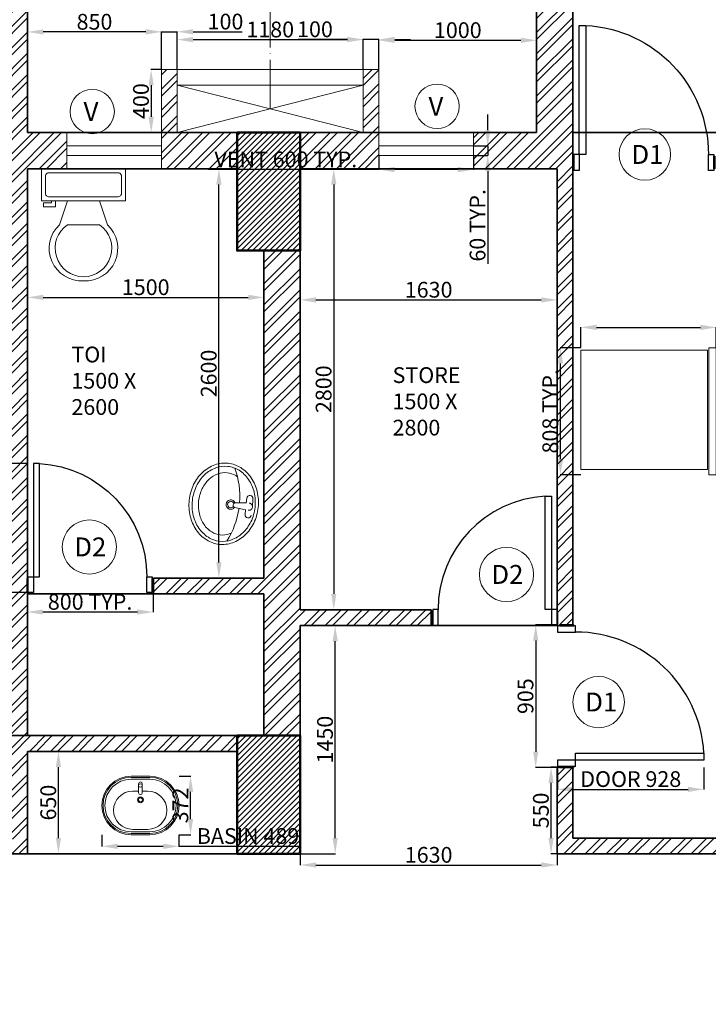
# Model space of a CAD drawing. Units: millimetres. Extents: x -3326 to 29338, y -16792 to 6002.
# Tile 9 of 21: x 3793 to 8162, y -3440 to 2813. Entities that reach past the tile are written whole.
import ezdxf

# ---------------------------------------------------------------- set-up
doc = ezdxf.new("R2010")
doc.units = ezdxf.units.MM
doc.header["$PDMODE"] = 35
doc.header["$PDSIZE"] = 5
doc.linetypes.add('ACAD_ISO04W100', pattern=[30, 24, -3, 0, -3])
for name, color, linetype, lineweight in [('A-ANNO-DIMS', 2, 'Continuous', 13), ('A-ANNO-SYMB', 7, 'Continuous', 18), ('A-AREA-IDEN', 7, 'Continuous', 18), ('A-COLS', 1, 'Continuous', 50), ('A-COLS-PATT', 251, 'Continuous', 13), ('A-DOOR', 3, 'Continuous', 25), ('A-EQPM', 9, 'Continuous', 18), ('A-FLOR-FIXT', 9, 'Continuous', 18), ('A-FLOR-SHFT', 8, 'Continuous', 18), ('A-GLAZ', 4, 'Continuous', 18), ('A-GRID', 8, 'ACAD_ISO04W100', 13), ('A-WALL', 7, 'Continuous', 35), ('A-WALL-PATT', 252, 'Continuous', 13)]:
    doc.layers.add(name, color=color, linetype=linetype, lineweight=lineweight)
doc.styles.get("Standard").update_dxf_attribs({"font": 'arial.ttf'})
doc.dimstyles.new('ISO-25', dxfattribs={"dimtxt": 100, "dimasz": 100, "dimexe": 1.25, "dimexo": 0.625, "dimtad": 1, "dimtxsty": 'Standard', "dimcen": 2.5, "dimadec": 0, "dimazin": 0, "dimtfac": 1, "dimtmove": 0, "dimatfit": 3, "dimfxl": 1, "dimarcsym": 0})
pattern_1 = [(45, (-10476.65, 1e-12), (-67.35192, 67.35192), []), (45, (-10431.74, 1e-12), (-67.35192, 67.35192), [])]

# ---------------------------------------------------------------- blocks, each defined once
blk = doc.blocks.new('A$C6ED17C1F')
for points in [[(793.9, 100), (720, 100), (720, 820), (760, 820), (760, 0), (793.9, 0)], [(6.1, 0), (40, 0), (40, 100), (6.1, 100)], [(6.1, 100), (6.1, 0)], [(793.9, 100), (793.9, 0)]]:
    blk.add_lwpolyline(points)
for points in [[(0, 10), (6.1, 10), (6.1, 90), (0, 90)], [(793.9, 10), (800, 10), (800, 90), (793.9, 90)]]:
    blk.add_lwpolyline(points, close=True)
blk.add_arc((761.2, 100), 721.2, 93.2732, 180)
blk = doc.blocks.new('A$C0CE462CD')
for p, q in [((860, 100), (860, 0)), ((860, 0), (893.9, 0))]:
    blk.add_line(p, q)
for points in [[(860, 100), (860, 920), (818.4, 920), (818.4, 100)], [(0, 10), (6.1, 10), (6.1, 90), (0, 90)], [(893.9, 10), (900, 10), (900, 90), (893.9, 90)]]:
    blk.add_lwpolyline(points, close=True)
for points in [[(6.1, 0), (40, 0), (40, 100), (6.1, 100)], [(6.1, 100), (6.1, 0)], [(860, 100), (893.9, 100), (893.9, 0)]]:
    blk.add_lwpolyline(points)
blk.add_arc((859.1, 101.9), 819.1, 92.8508, 180.13091)
blk = doc.blocks.new('*U5')
for p, q in [((9.5, -6), (9.5, -2)), ((-10, -8.5), (-8, -8.5)), ((-10, -9.5), (-10, -8.5)), ((-7, -9.5), (-10, -9.5)), ((-8, -8.5), (-8, -8)), ((-7, -8), (-7, -9.5)), ((-4, -8), (-6, -14)), ((4, -8), (6, -14)), ((4, -14), (-4, -14))]:
    blk.add_line(p, q)
blk.add_lwpolyline([(10.5, -8), (10.5, 0), (-10.5, 0), (-10.5, -8)], close=True)
for points in [[(-9.5, -2), (-9.5, -6)], [(8.5, -1), (-8.5, -1)], [(-8.5, -7), (8.5, -7)]]:
    blk.add_lwpolyline(points)
for centre, radius, start, end in [((-8.625, -1.875), 0.8839, 81.8699, 188.1301), ((8.625, -1.875), 0.8839, 351.8699, 98.1301), ((-8.625, -6.125), 0.8839, 171.869898, 278.1301), ((8.625, -6.125), 0.8839, 261.8699, 8.1301), ((-0.4772, -19.9188), 8.0953, 133.01722, 273.38), ((0.0374, -19.8731), 7.127, 124.50543, 269.7), ((-0.0373, -19.8731), 7.127, 270.3, 55.4946), ((0.4773, -19.9188), 8.0953, 266.62, 46.9828)]:
    blk.add_arc(centre, radius, start, end)
blk = doc.blocks.new('A$C6B943AC5')
for p, q in [((0.207, 0.401), (0.2589, 0.4042)), ((0.2071, 0.362), (0.2386, 0.3621)), ((0.2361, 0.3625), (0.2439, 0.2926)), ((0.2809, 0.3627), (0.2736, 0.2927)), ((0.3111, 0.3624), (0.2796, 0.3623))]:
    blk.add_line(p, q)
for points in [[(0.518, 0.2209, -0.113917), (0.4993, 0.1385, -0.1036), (0.4427, 0.0651, -0.091717), (0.3606, 0.0176, -0.084781), (0.2598, 0, -0.084781), (0.1587, 0.0169, -0.091717), (0.0764, 0.0638, -0.1036), (0.0193, 0.1368, -0.113917), (0, 0.2191, -0.113917), (0.0187, 0.3015, -0.1036), (0.0753, 0.3749, -0.091717), (0.1574, 0.4224, -0.084781), (0.2582, 0.44, -0.084781), (0.3592, 0.4231, -0.091717), (0.4416, 0.3762, -0.1036), (0.4987, 0.3032, -0.113917)], [(0.498, 0.2208, -0.113917), (0.4813, 0.1472, -0.1036), (0.4297, 0.0803, -0.091717), (0.3539, 0.0364, -0.084781), (0.2597, 0.02, -0.084781), (0.1653, 0.0358, -0.091717), (0.0893, 0.0791, -0.1036), (0.0372, 0.1457, -0.113917), (0.02, 0.2192, -0.113917), (0.0367, 0.2928, -0.1036), (0.0883, 0.3597, -0.091717), (0.1641, 0.4036, -0.084781), (0.2583, 0.42, -0.084781), (0.3527, 0.4042, -0.091717), (0.4287, 0.3609, -0.1036), (0.4808, 0.2943, -0.113917)]]:
    blk.add_lwpolyline(points, format="xyb", close=True)
for points in [[(0.458, 0.2207, -0.113917), (0.4453, 0.1646, -0.1036), (0.4037, 0.1107, -0.091717), (0.3405, 0.0741, -0.084781), (0.2595, 0.06, -0.084781), (0.1785, 0.0736, -0.091717), (0.1151, 0.1097, -0.1036), (0.0731, 0.1633, -0.113917), (0.06, 0.2193, -0.113917), (0.0727, 0.2754, -0.020517), (0.0792, 0.2874, -0.091717)], [(0.4384, 0.2886, -0.020517), (0.4449, 0.2767, -0.113917), (0.458, 0.2207, -0.113917)]]:
    blk.add_lwpolyline(points, format="xyb")
for centre, radius, start, end in [((0.207, 0.3815), 0.0195, 90.19698, 270.19698), ((0.259, 0.3817), 0.0225, 354.08148, 186.31248), ((0.311, 0.3819), 0.0195, 270.19698, 90.19698), ((0.2604, -0.2004), 0.5204, 92.15427, 116.77617), ((0.2604, -0.2004), 0.5204, 63.61779, 88.23969), ((0.2588, 0.265), 0.03, 119.152, 61.24195), ((0.2588, 0.265), 0.02, 116.58131, 63.81265), ((0.2587, 0.295), 0.015, 189.39225, 351.00171)]:
    blk.add_arc(centre, radius, start, end)
blk = doc.blocks.new('A$C6AF055E0')
for p, q in [((0.1999, 0.245), (0.1225, 0.245)), ((0.1999, 0.24), (0.1225, 0.24)), ((0.1999, 0.2325), (0.1225, 0.2325)), ((0.1537, 0.1758), (0.1537, 0.2135)), ((0.1687, 0.2135), (0.1687, 0.1758)), ((0.129, 0.1825), (0.1537, 0.1825)), ((0.1687, 0.1825), (0.1919, 0.1825)), ((0.1225, 0.0125), (0.1999, 0.0125)), ((0.1225, 0.005), (0.1999, 0.005)), ((0.1225, 0), (0.1999, 0)), ((0.129, 0.0225), (0.1919, 0.0225))]:
    blk.add_line(p, q)
for centre, radius in [((0.1612, 0.206), 0.0075), ((0.1612, 0.1463), 0.0125), ((0.1612, 0.1463), 0.0085)]:
    blk.add_circle(centre, radius)
for centre, radius, start, end in [((0.1225, 0.1225), 0.1225, 90, 270), ((0.1225, 0.1225), 0.1175, 90, 270), ((0.1225, 0.1225), 0.11, 90, 270), ((0.1612, 0.2135), 0.0075, 0, 180), ((0.1999, 0.1225), 0.1225, 270, 90), ((0.1999, 0.1225), 0.1175, 270, 90), ((0.1999, 0.1225), 0.11, 270, 90), ((0.129, 0.1025), 0.08, 90, 270), ((0.1612, 0.1758), 0.0075, 180, 0), ((0.1919, 0.1025), 0.08, 270, 90)]:
    blk.add_arc(centre, radius, start, end)
blk = doc.blocks.new('*D128')
at = {"layer": 'A-ANNO-DIMS', "color": 0, "lineweight": -2, "transparency": 16777216}
for p, q in [((5572.3, 1033.9), (5572.3, 1034.6)), ((5672.3, 1033.3), (7102.3, 1033.3)), ((7202.3, 1033.9), (7202.3, 1034.6))]:
    blk.add_line(p, q, dxfattribs=at)
at = {"layer": 'A-ANNO-DIMS', "color": 0, "transparency": 16777216}
for points in [[(5672.3, 1050), (5672.3, 1016.6), (5572.3, 1033.3)], [(7102.3, 1050), (7102.3, 1016.6), (7202.3, 1033.3)]]:
    blk.add_solid(points, dxfattribs=at)
at = {"layer": 'Defpoints', "color": 0, "transparency": 16777216}
for p in [(5572.3, 1033.3), (7202.3, 1033.3), (7202.3, 1033.3)]:
    blk.add_point(p, dxfattribs=at)
at = {"layer": 'A-ANNO-DIMS', "color": 0, "transparency": 16777216, "insert": (6387.3, 1085), "char_height": 100, "attachment_point": 5}
blk.add_mtext('1630', dxfattribs=at)
blk = doc.blocks.new('*D129')
at = {"layer": 'A-ANNO-DIMS', "color": 0, "lineweight": -2, "transparency": 16777216}
for p, q in [((5572.9, 1866), (5786.7, 1866)), ((5785.5, 1766), (5785.5, -834)), ((5572.9, -934), (5786.7, -934))]:
    blk.add_line(p, q, dxfattribs=at)
at = {"layer": 'A-ANNO-DIMS', "color": 0, "transparency": 16777216}
for points in [[(5768.8, 1766), (5802.1, 1766), (5785.5, 1866)], [(5768.8, -834), (5802.1, -834), (5785.5, -934)]]:
    blk.add_solid(points, dxfattribs=at)
at = {"layer": 'Defpoints', "color": 0, "transparency": 16777216}
for p in [(5572.3, 1866), (5572.3, -934), (5785.5, -934)]:
    blk.add_point(p, dxfattribs=at)
at = {"layer": 'A-ANNO-DIMS', "color": 0, "transparency": 16777216, "insert": (5733.8, 466), "char_height": 100, "attachment_point": 5, "rotation": 90}
blk.add_mtext('2800', dxfattribs=at)
blk = doc.blocks.new('*D130')
at = {"layer": 'A-ANNO-DIMS', "color": 0, "lineweight": -2, "transparency": 16777216}
for p, q in [((3842.3, 1103.3), (3842.3, 1048.1)), ((5342.3, 1103.3), (5342.3, 1048.1)), ((3942.3, 1049.4), (5242.3, 1049.4))]:
    blk.add_line(p, q, dxfattribs=at)
at = {"layer": 'A-ANNO-DIMS', "color": 0, "transparency": 16777216}
for points in [[(3942.3, 1066), (3942.3, 1032.7), (3842.3, 1049.4)], [(5242.3, 1066), (5242.3, 1032.7), (5342.3, 1049.4)]]:
    blk.add_solid(points, dxfattribs=at)
at = {"layer": 'Defpoints', "color": 0, "transparency": 16777216}
for p in [(3842.3, 1103.9), (5342.3, 1103.9), (5342.3, 1049.4)]:
    blk.add_point(p, dxfattribs=at)
at = {"layer": 'A-ANNO-DIMS', "color": 0, "transparency": 16777216, "insert": (4592.3, 1101.1), "char_height": 100, "attachment_point": 5}
blk.add_mtext('1500', dxfattribs=at)
blk = doc.blocks.new('*D131')
at = {"layer": 'A-ANNO-DIMS', "color": 0, "lineweight": -2, "transparency": 16777216}
for p, q in [((5171.7, 1866), (5055.3, 1866)), ((5056.6, -634), (5056.6, 1766)), ((5341.7, -734), (5055.3, -734))]:
    blk.add_line(p, q, dxfattribs=at)
at = {"layer": 'A-ANNO-DIMS', "color": 0, "transparency": 16777216}
for points in [[(5039.9, 1766), (5073.2, 1766), (5056.6, 1866)], [(5039.9, -634), (5073.2, -634), (5056.6, -734)]]:
    blk.add_solid(points, dxfattribs=at)
at = {"layer": 'Defpoints', "color": 0, "transparency": 16777216}
for p in [(5056.6, 1866), (5172.3, 1866), (5342.3, -734)]:
    blk.add_point(p, dxfattribs=at)
at = {"layer": 'A-ANNO-DIMS', "color": 0, "transparency": 16777216, "insert": (5004.9, 566), "char_height": 100, "attachment_point": 5, "rotation": 90}
blk.add_mtext('2600', dxfattribs=at)
blk = doc.blocks.new('*D132')
at = {"layer": 'A-ANNO-DIMS', "color": 0, "lineweight": -2, "transparency": 16777216}
for p, q in [((5572.9, -1034), (5795.7, -1034)), ((5794.4, -2384), (5794.4, -1134)), ((5572.9, -2484), (5795.7, -2484))]:
    blk.add_line(p, q, dxfattribs=at)
at = {"layer": 'A-ANNO-DIMS', "color": 0, "transparency": 16777216}
for points in [[(5777.8, -1134), (5811.1, -1134), (5794.4, -1034)], [(5777.8, -2384), (5811.1, -2384), (5794.4, -2484)]]:
    blk.add_solid(points, dxfattribs=at)
at = {"layer": 'Defpoints', "color": 0, "transparency": 16777216}
for p in [(5572.3, -1034), (5794.4, -1034), (5572.3, -2484)]:
    blk.add_point(p, dxfattribs=at)
at = {"layer": 'A-ANNO-DIMS', "color": 0, "transparency": 16777216, "insert": (5742.8, -1759), "char_height": 100, "attachment_point": 5, "rotation": 90}
blk.add_mtext('1450', dxfattribs=at)
blk = doc.blocks.new('*D133')
at = {"layer": 'A-ANNO-DIMS', "color": 0, "lineweight": -2, "transparency": 16777216}
for p, q in [((7201.7, -1934), (7162.8, -1934)), ((7164.1, -2384), (7164.1, -2034)), ((7201.7, -2484), (7162.8, -2484))]:
    blk.add_line(p, q, dxfattribs=at)
at = {"layer": 'A-ANNO-DIMS', "color": 0, "transparency": 16777216}
for points in [[(7147.4, -2034), (7180.7, -2034), (7164.1, -1934)], [(7147.4, -2384), (7180.7, -2384), (7164.1, -2484)]]:
    blk.add_solid(points, dxfattribs=at)
at = {"layer": 'Defpoints', "color": 0, "transparency": 16777216}
for p in [(7164.1, -1934), (7202.3, -1934), (7202.3, -2484)]:
    blk.add_point(p, dxfattribs=at)
at = {"layer": 'A-ANNO-DIMS', "color": 0, "transparency": 16777216, "insert": (7112.4, -2209), "char_height": 100, "attachment_point": 5, "rotation": 90}
blk.add_mtext('550', dxfattribs=at)
blk = doc.blocks.new('*D134')
at = {"layer": 'A-ANNO-DIMS', "color": 0, "lineweight": -2, "transparency": 16777216}
for p, q in [((5572.3, -2484.6), (5572.3, -2556.8)), ((7202.3, -2484.6), (7202.3, -2556.8)), ((5672.3, -2555.5), (7102.3, -2555.5))]:
    blk.add_line(p, q, dxfattribs=at)
at = {"layer": 'A-ANNO-DIMS', "color": 0, "transparency": 16777216}
for points in [[(5672.3, -2538.9), (5672.3, -2572.2), (5572.3, -2555.5)], [(7102.3, -2538.9), (7102.3, -2572.2), (7202.3, -2555.5)]]:
    blk.add_solid(points, dxfattribs=at)
at = {"layer": 'Defpoints', "color": 0, "transparency": 16777216}
for p in [(5572.3, -2484), (7202.3, -2484), (7202.3, -2555.5)]:
    blk.add_point(p, dxfattribs=at)
at = {"layer": 'A-ANNO-DIMS', "color": 0, "transparency": 16777216, "insert": (6387.3, -2503.8), "char_height": 100, "attachment_point": 5}
blk.add_mtext('1630', dxfattribs=at)
blk = doc.blocks.new('*D135')
at = {"layer": 'A-ANNO-DIMS', "color": 0, "lineweight": -2, "transparency": 16777216}
for p, q in [((3842.9, -1834), (4039.8, -1834)), ((4038.5, -2384), (4038.5, -1934)), ((3842.9, -2484), (4039.8, -2484))]:
    blk.add_line(p, q, dxfattribs=at)
at = {"layer": 'A-ANNO-DIMS', "color": 0, "transparency": 16777216}
for points in [[(4021.9, -1934), (4055.2, -1934), (4038.5, -1834)], [(4021.9, -2384), (4055.2, -2384), (4038.5, -2484)]]:
    blk.add_solid(points, dxfattribs=at)
at = {"layer": 'Defpoints', "color": 0, "transparency": 16777216}
for p in [(3842.3, -1834), (4038.5, -1834), (3842.3, -2484)]:
    blk.add_point(p, dxfattribs=at)
at = {"layer": 'A-ANNO-DIMS', "color": 0, "transparency": 16777216, "insert": (3986.9, -2159), "char_height": 100, "attachment_point": 5, "rotation": 90}
blk.add_mtext('650', dxfattribs=at)
blk = doc.blocks.new('*D145')
at = {"layer": 'A-ANNO-DIMS', "color": 0, "lineweight": -2, "transparency": 16777216}
for p, q in [((4792.3, 2496.7), (4792.3, 2687.3)), ((4892.3, 2686.1), (5872.3, 2686.1)), ((5972.3, 2496.7), (5972.3, 2687.3))]:
    blk.add_line(p, q, dxfattribs=at)
at = {"layer": 'A-ANNO-DIMS', "color": 0, "transparency": 16777216}
for points in [[(4892.3, 2702.8), (4892.3, 2669.4), (4792.3, 2686.1)], [(5872.3, 2702.8), (5872.3, 2669.4), (5972.3, 2686.1)]]:
    blk.add_solid(points, dxfattribs=at)
at = {"layer": 'Defpoints', "color": 0, "transparency": 16777216}
for p in [(5972.3, 2686.1), (4792.3, 2496), (5972.3, 2496)]:
    blk.add_point(p, dxfattribs=at)
at = {"layer": 'A-ANNO-DIMS', "color": 0, "transparency": 16777216, "insert": (5382.3, 2737.8), "char_height": 100, "attachment_point": 5}
blk.add_mtext('1180', dxfattribs=at)
blk = doc.blocks.new('*D146')
at = {"layer": 'A-ANNO-DIMS', "color": 0, "lineweight": -2, "transparency": 16777216}
for p, q in [((4592.3, 2736.2), (4492.3, 2736.2)), ((4692.3, 2496.7), (4692.3, 2737.4)), ((4692.3, 2736.2), (4792.3, 2736.2)), ((4792.3, 2496.7), (4792.3, 2737.4)), ((4892.3, 2736.2), (5204.7, 2736.2))]:
    blk.add_line(p, q, dxfattribs=at)
at = {"layer": 'A-ANNO-DIMS', "color": 0, "transparency": 16777216}
for points in [[(4592.3, 2752.9), (4592.3, 2719.5), (4692.3, 2736.2)], [(4892.3, 2752.9), (4892.3, 2719.5), (4792.3, 2736.2)]]:
    blk.add_solid(points, dxfattribs=at)
at = {"layer": 'Defpoints', "color": 0, "transparency": 16777216}
for p in [(4792.3, 2736.2), (4692.3, 2496), (4792.3, 2496)]:
    blk.add_point(p, dxfattribs=at)
at = {"layer": 'A-ANNO-DIMS', "color": 0, "transparency": 16777216, "insert": (5098.5, 2787.9), "char_height": 100, "attachment_point": 5}
blk.add_mtext('100', dxfattribs=at)
blk = doc.blocks.new('*D147')
at = {"layer": 'A-ANNO-DIMS', "color": 0, "lineweight": -2, "transparency": 16777216}
for p, q in [((5872.3, 2687.3), (5559.9, 2687.3)), ((5972.3, 2496.7), (5972.3, 2688.6)), ((6072.3, 2687.3), (5972.3, 2687.3)), ((6072.3, 2496.7), (6072.3, 2688.6)), ((6172.3, 2687.3), (6272.3, 2687.3))]:
    blk.add_line(p, q, dxfattribs=at)
at = {"layer": 'A-ANNO-DIMS', "color": 0, "transparency": 16777216}
for points in [[(5872.3, 2704), (5872.3, 2670.7), (5972.3, 2687.3)], [(6172.3, 2704), (6172.3, 2670.7), (6072.3, 2687.3)]]:
    blk.add_solid(points, dxfattribs=at)
at = {"layer": 'Defpoints', "color": 0, "transparency": 16777216}
for p in [(5972.3, 2687.3), (5972.3, 2496), (6072.3, 2496)]:
    blk.add_point(p, dxfattribs=at)
at = {"layer": 'A-ANNO-DIMS', "color": 0, "transparency": 16777216, "insert": (5666.1, 2739), "char_height": 100, "attachment_point": 5}
blk.add_mtext('100', dxfattribs=at)
blk = doc.blocks.new('*D148')
at = {"layer": 'A-ANNO-DIMS', "color": 0, "lineweight": -2, "transparency": 16777216}
for p, q in [((6072.3, 2593.3), (6072.3, 2683)), ((6172.3, 2681.8), (6972.3, 2681.8)), ((7072.3, 2593.3), (7072.3, 2683))]:
    blk.add_line(p, q, dxfattribs=at)
at = {"layer": 'A-ANNO-DIMS', "color": 0, "transparency": 16777216}
for points in [[(6172.3, 2698.4), (6172.3, 2665.1), (6072.3, 2681.8)], [(6972.3, 2698.4), (6972.3, 2665.1), (7072.3, 2681.8)]]:
    blk.add_solid(points, dxfattribs=at)
at = {"layer": 'Defpoints', "color": 0, "transparency": 16777216}
for p in [(7072.3, 2681.8), (6072.3, 2592.6), (7072.3, 2592.6)]:
    blk.add_point(p, dxfattribs=at)
at = {"layer": 'A-ANNO-DIMS', "color": 0, "transparency": 16777216, "insert": (6572.3, 2733.4), "char_height": 100, "attachment_point": 5}
blk.add_mtext('1000', dxfattribs=at)
blk = doc.blocks.new('*D149')
at = {"layer": 'A-ANNO-DIMS', "color": 0, "lineweight": -2, "transparency": 16777216}
for p, q in [((3842.3, 2617.7), (3842.3, 2736.3)), ((4592.3, 2735), (3942.3, 2735)), ((4692.3, 2617.7), (4692.3, 2736.3))]:
    blk.add_line(p, q, dxfattribs=at)
at = {"layer": 'A-ANNO-DIMS', "color": 0, "transparency": 16777216}
for points in [[(3942.3, 2751.7), (3942.3, 2718.4), (3842.3, 2735)], [(4592.3, 2751.7), (4592.3, 2718.4), (4692.3, 2735)]]:
    blk.add_solid(points, dxfattribs=at)
at = {"layer": 'Defpoints', "color": 0, "transparency": 16777216}
for p in [(3842.3, 2735), (3842.3, 2617.1), (4692.3, 2617.1)]:
    blk.add_point(p, dxfattribs=at)
at = {"layer": 'A-ANNO-DIMS', "color": 0, "transparency": 16777216, "insert": (4267.3, 2786.7), "char_height": 100, "attachment_point": 5}
blk.add_mtext('850', dxfattribs=at)
blk = doc.blocks.new('*D150')
at = {"layer": 'A-ANNO-DIMS', "color": 0, "lineweight": -2, "transparency": 16777216}
for p, q in [((4691.7, 2496), (4625.5, 2496)), ((4626.8, 2396), (4626.8, 2196)), ((4691.7, 2096), (4625.5, 2096))]:
    blk.add_line(p, q, dxfattribs=at)
at = {"layer": 'A-ANNO-DIMS', "color": 0, "transparency": 16777216}
for points in [[(4610.1, 2396), (4643.5, 2396), (4626.8, 2496)], [(4610.1, 2196), (4643.5, 2196), (4626.8, 2096)]]:
    blk.add_solid(points, dxfattribs=at)
at = {"layer": 'Defpoints', "color": 0, "transparency": 16777216}
for p in [(4692.3, 2496), (4626.8, 2096), (4692.3, 2096)]:
    blk.add_point(p, dxfattribs=at)
at = {"layer": 'A-ANNO-DIMS', "color": 0, "transparency": 16777216, "insert": (4575.1, 2296), "char_height": 100, "attachment_point": 5, "rotation": 90}
blk.add_mtext('400', dxfattribs=at)
blk = doc.blocks.new('REFRIGERATOR-PLAN')
for points in [[(0, 791.3), (804.9, 791.3), (804.9, 34.9), (0, 34.9)], [(812.5, 807.8), (859.3, 807.8), (859.3, 0), (812.5, 0)]]:
    blk.add_lwpolyline(points, close=True)
blk = doc.blocks.new('TAG-D1')
blk.add_circle((163.3, 163.3), 163.3)
at = {"insert": (78, 223.5), "char_height": 120, "attachment_point": 1}
blk.add_mtext_dynamic_manual_height_columns('D1', width=137.943, gutter_width=12.5, heights=[0], dxfattribs=at)
blk = doc.blocks.new('TAG-D2')
blk.add_circle((172, 172), 172)
at = {"insert": (75.7, 232.2), "char_height": 120, "attachment_point": 1}
blk.add_mtext_dynamic_manual_height_columns('D2', width=130.724, gutter_width=12.5, heights=[0], dxfattribs=at)
blk = doc.blocks.new('TAG-V')
blk.add_circle((140.7, 140.7), 140.7)
at = {"insert": (85.8, 200.7), "char_height": 120, "attachment_point": 1}
blk.add_mtext_dynamic_manual_height_columns('V', width=129.836, gutter_width=12.5, heights=[0], dxfattribs=at)
blk = doc.blocks.new('GLAZ-600x60')
for p, q in [((0, 60), (600, 60)), ((0, 0), (600, 0))]:
    blk.add_line(p, q)
blk = doc.blocks.new('*D197')
at = {"layer": 'A-ANNO-DIMS', "color": 0, "lineweight": -2, "transparency": 16777216}
for p, q in [((3716.3, -5.8), (3716.3, 1112.9)), ((3838.6, -5.8), (3715, -5.8)), ((3716.3, -725.8), (3716.3, -105.8)), ((3838.6, -825.8), (3715, -825.8))]:
    blk.add_line(p, q, dxfattribs=at)
at = {"layer": 'A-ANNO-DIMS', "color": 0, "transparency": 16777216}
for points in [[(3699.6, -105.8), (3732.9, -105.8), (3716.3, -5.8)], [(3699.6, -725.8), (3732.9, -725.8), (3716.3, -825.8)]]:
    blk.add_solid(points, dxfattribs=at)
at = {"layer": 'Defpoints', "color": 0, "transparency": 16777216}
for p in [(3716.3, -5.8), (3839.3, -5.8), (3839.3, -825.8)]:
    blk.add_point(p, dxfattribs=at)
at = {"layer": 'A-ANNO-DIMS', "color": 0, "transparency": 16777216, "insert": (3663.9, 603.5), "char_height": 100, "attachment_point": 5, "rotation": 90}
blk.add_mtext('DOOR 820 TYP.', dxfattribs=at)
blk = doc.blocks.new('*D198')
at = {"layer": 'A-ANNO-DIMS', "color": 0, "lineweight": -2, "transparency": 16777216}
for p, q in [((3839.3, -826.4), (3839.3, -950)), ((4639.3, -826.4), (4639.3, -950)), ((4539.3, -948.8), (3939.3, -948.8))]:
    blk.add_line(p, q, dxfattribs=at)
at = {"layer": 'A-ANNO-DIMS', "color": 0, "transparency": 16777216}
for points in [[(3939.3, -932.1), (3939.3, -965.5), (3839.3, -948.8)], [(4539.3, -932.1), (4539.3, -965.5), (4639.3, -948.8)]]:
    blk.add_solid(points, dxfattribs=at)
at = {"layer": 'Defpoints', "color": 0, "transparency": 16777216}
for p in [(3839.3, -825.8), (4639.3, -825.8), (3839.3, -948.8)]:
    blk.add_point(p, dxfattribs=at)
at = {"layer": 'A-ANNO-DIMS', "color": 0, "transparency": 16777216, "insert": (4239.3, -897.1), "char_height": 100, "attachment_point": 5}
blk.add_mtext('800 TYP.', dxfattribs=at)
blk = doc.blocks.new('*D199')
at = {"layer": 'A-ANNO-DIMS', "color": 0, "lineweight": -2, "transparency": 16777216}
for p, q in [((7205.7, -1936.4), (7205.7, -2076.2)), ((8133.7, -1936.4), (8133.7, -2076.2)), ((7305.7, -2075), (8033.7, -2075))]:
    blk.add_line(p, q, dxfattribs=at)
at = {"layer": 'A-ANNO-DIMS', "color": 0, "transparency": 16777216}
for points in [[(7305.7, -2058.3), (7305.7, -2091.6), (7205.7, -2075)], [(8033.7, -2058.3), (8033.7, -2091.6), (8133.7, -2075)]]:
    blk.add_solid(points, dxfattribs=at)
at = {"layer": 'Defpoints', "color": 0, "transparency": 16777216}
for p in [(7205.7, -1935.8), (8133.7, -1935.8), (8133.7, -2075)]:
    blk.add_point(p, dxfattribs=at)
at = {"layer": 'A-ANNO-DIMS', "color": 0, "transparency": 16777216, "insert": (7669.7, -2022.6), "char_height": 100, "attachment_point": 5}
blk.add_mtext('DOOR 928', dxfattribs=at)
blk = doc.blocks.new('*D200')
at = {"layer": 'A-ANNO-DIMS', "color": 0, "lineweight": -2, "transparency": 16777216}
for p, q in [((7205.1, -1030.4), (7065.3, -1030.4)), ((7066.5, -1130.4), (7066.5, -1835.8)), ((7205.1, -1935.8), (7065.3, -1935.8))]:
    blk.add_line(p, q, dxfattribs=at)
at = {"layer": 'A-ANNO-DIMS', "color": 0, "transparency": 16777216}
for points in [[(7049.8, -1130.4), (7083.2, -1130.4), (7066.5, -1030.4)], [(7049.8, -1835.8), (7083.2, -1835.8), (7066.5, -1935.8)]]:
    blk.add_solid(points, dxfattribs=at)
at = {"layer": 'Defpoints', "color": 0, "transparency": 16777216}
for p in [(7205.7, -1030.4), (7066.5, -1935.8), (7205.7, -1935.8)]:
    blk.add_point(p, dxfattribs=at)
at = {"layer": 'A-ANNO-DIMS', "color": 0, "transparency": 16777216, "insert": (7014.8, -1483.1), "char_height": 100, "attachment_point": 5, "rotation": 90}
blk.add_mtext('905', dxfattribs=at)
blk = doc.blocks.new('*D209')
at = {"layer": 'A-ANNO-DIMS', "color": 0, "lineweight": -2, "transparency": 16777216}
for p, q in [((6072.3, 1950.4), (6072.3, 1859.8)), ((6672.3, 1950.4), (6672.3, 1859.8)), ((6072.3, 1861), (4990, 1861)), ((6572.3, 1861), (6172.3, 1861))]:
    blk.add_line(p, q, dxfattribs=at)
at = {"layer": 'A-ANNO-DIMS', "color": 0, "transparency": 16777216}
for points in [[(6172.3, 1877.7), (6172.3, 1844.4), (6072.3, 1861)], [(6572.3, 1877.7), (6572.3, 1844.4), (6672.3, 1861)]]:
    blk.add_solid(points, dxfattribs=at)
at = {"layer": 'Defpoints', "color": 0, "transparency": 16777216}
for p in [(6072.3, 1951), (6672.3, 1951), (6072.3, 1861)]:
    blk.add_point(p, dxfattribs=at)
at = {"layer": 'A-ANNO-DIMS', "color": 0, "transparency": 16777216, "insert": (5481.2, 1912.7), "char_height": 100, "attachment_point": 5}
blk.add_mtext('VENT 600 TYP.', dxfattribs=at)
blk = doc.blocks.new('*D210')
at = {"layer": 'A-ANNO-DIMS', "color": 0, "lineweight": -2, "transparency": 16777216}
for p, q in [((6762.3, 2111), (6762.3, 2211)), ((6672.9, 2011), (6763.6, 2011)), ((6762.3, 2011), (6762.3, 1951)), ((6672.9, 1951), (6763.6, 1951)), ((6762.3, 1851), (6762.3, 1262.5))]:
    blk.add_line(p, q, dxfattribs=at)
at = {"layer": 'A-ANNO-DIMS', "color": 0, "transparency": 16777216}
for points in [[(6745.6, 2111), (6779, 2111), (6762.3, 2011)], [(6745.6, 1851), (6779, 1851), (6762.3, 1951)]]:
    blk.add_solid(points, dxfattribs=at)
at = {"layer": 'Defpoints', "color": 0, "transparency": 16777216}
for p in [(6672.3, 2011), (6672.3, 1951), (6762.3, 1951)]:
    blk.add_point(p, dxfattribs=at)
at = {"layer": 'A-ANNO-DIMS', "color": 0, "transparency": 16777216, "insert": (6710.6, 1506.8), "char_height": 100, "attachment_point": 5, "rotation": 90}
blk.add_mtext('60 TYP.', dxfattribs=at)
blk = doc.blocks.new('*D217')
at = {"layer": 'A-ANNO-DIMS', "color": 0, "lineweight": -2, "transparency": 16777216}
for p, q in [((4314.1, -2363.8), (4314.1, -2437.9)), ((4803.4, -2363.8), (4803.4, -2437.9)), ((4414.1, -2436.6), (4703.4, -2436.6)), ((4803.4, -2436.6), (5579.4, -2436.6))]:
    blk.add_line(p, q, dxfattribs=at)
at = {"layer": 'A-ANNO-DIMS', "color": 0, "transparency": 16777216}
for points in [[(4414.1, -2419.9), (4414.1, -2453.3), (4314.1, -2436.6)], [(4703.4, -2419.9), (4703.4, -2453.3), (4803.4, -2436.6)]]:
    blk.add_solid(points, dxfattribs=at)
at = {"layer": 'Defpoints', "color": 0, "transparency": 16777216}
for p in [(4314.1, -2363.2), (4803.4, -2363.2), (4803.4, -2436.6)]:
    blk.add_point(p, dxfattribs=at)
at = {"layer": 'A-ANNO-DIMS', "color": 0, "transparency": 16777216, "insert": (5241.4, -2384.3), "char_height": 100, "attachment_point": 5}
blk.add_mtext('BASIN 489', dxfattribs=at)
blk = doc.blocks.new('*D218')
at = {"layer": 'A-ANNO-DIMS', "color": 0, "lineweight": -2, "transparency": 16777216}
for p, q in [((4804, -1991.4), (4878.1, -1991.4)), ((4876.8, -2263.2), (4876.8, -2091.4)), ((4804, -2363.2), (4878.1, -2363.2))]:
    blk.add_line(p, q, dxfattribs=at)
at = {"layer": 'A-ANNO-DIMS', "color": 0, "transparency": 16777216}
for points in [[(4860.2, -2091.4), (4893.5, -2091.4), (4876.8, -1991.4)], [(4860.2, -2263.2), (4893.5, -2263.2), (4876.8, -2363.2)]]:
    blk.add_solid(points, dxfattribs=at)
at = {"layer": 'Defpoints', "color": 0, "transparency": 16777216}
for p in [(4803.4, -1991.4), (4876.8, -1991.4), (4803.4, -2363.2)]:
    blk.add_point(p, dxfattribs=at)
at = {"layer": 'A-ANNO-DIMS', "color": 0, "transparency": 16777216, "insert": (4825.1, -2177.3), "char_height": 100, "attachment_point": 5, "rotation": 90}
blk.add_mtext('372', dxfattribs=at)
blk = doc.blocks.new('*D233')
at = {"layer": 'A-ANNO-DIMS', "color": 0, "lineweight": -2, "transparency": 16777216}
for p, q in [((7352.6, 730.5), (7352.6, 860.1)), ((7452.6, 858.8), (8111.9, 858.8)), ((8211.9, 730.5), (8211.9, 860.1)), ((8211.9, 858.8), (9438.5, 858.8))]:
    blk.add_line(p, q, dxfattribs=at)
at = {"layer": 'A-ANNO-DIMS', "color": 0, "transparency": 16777216}
for points in [[(7452.6, 875.5), (7452.6, 842.1), (7352.6, 858.8)], [(8111.9, 875.5), (8111.9, 842.1), (8211.9, 858.8)]]:
    blk.add_solid(points, dxfattribs=at)
at = {"layer": 'Defpoints', "color": 0, "transparency": 16777216}
for p in [(8211.9, 858.8), (7352.6, 729.9), (8211.9, 729.9)]:
    blk.add_point(p, dxfattribs=at)
at = {"layer": 'A-ANNO-DIMS', "color": 0, "transparency": 16777216, "insert": (8875.2, 911.1), "char_height": 100, "attachment_point": 5}
blk.add_mtext('FRIDGE 859 TYP.', dxfattribs=at)
blk = doc.blocks.new('*D234')
at = {"layer": 'A-ANNO-DIMS', "color": 0, "lineweight": -2, "transparency": 16777216}
for p, q in [((7352, 729.9), (7222.5, 729.9)), ((7223.7, 22.1), (7223.7, 629.9)), ((7352, -77.9), (7222.5, -77.9))]:
    blk.add_line(p, q, dxfattribs=at)
at = {"layer": 'A-ANNO-DIMS', "color": 0, "transparency": 16777216}
for points in [[(7207.1, 629.9), (7240.4, 629.9), (7223.7, 729.9)], [(7207.1, 22.1), (7240.4, 22.1), (7223.7, -77.9)]]:
    blk.add_solid(points, dxfattribs=at)
at = {"layer": 'Defpoints', "color": 0, "transparency": 16777216}
for p in [(7223.7, 729.9), (7352.6, 729.9), (7352.6, -77.9)]:
    blk.add_point(p, dxfattribs=at)
at = {"layer": 'A-ANNO-DIMS', "color": 0, "transparency": 16777216, "insert": (7172, 326), "char_height": 100, "attachment_point": 5, "rotation": 90}
blk.add_mtext('808 TYP.', dxfattribs=at)

msp = doc.modelspace()

# ---------------------------------------------------------------- hatches: boundary and pattern name
at = {"layer": 'A-COLS-PATT'}
h = msp.add_hatch(dxfattribs=at)
h.set_pattern_fill('ANSI31', color=256, scale=8)
h.set_pattern_definition([(45, (-36866.33, 12265.585), (-17.960512, 17.960512), [])])
h.paths.add_polyline_path([(5572.301, 2096.048), (5172.301, 2096.048), (5172.301, 1346.048), (5572.301, 1346.048)])
h = msp.add_hatch(dxfattribs=at)
h.set_pattern_fill('ANSI31', color=256, scale=8)
h.set_pattern_definition([(45, (-36866.33, 8435.585), (-17.960512, 17.960512), [])])
h.paths.add_polyline_path([(5572.301, -1733.952), (5172.301, -1733.952), (5172.301, -2483.952), (5572.301, -2483.952)])
at = {"layer": 'A-WALL-PATT'}
h = msp.add_hatch(dxfattribs=at)
h.set_pattern_fill('ANSI32', color=256, scale=10)
h.set_pattern_definition(pattern_1)
h.paths.add_polyline_path([(2842.301, -2383.952), (-215.519, -2383.952), (-215.519, -2483.952), (1282.301, -2483.952), (1282.301, -2683.952), (1413.549, -2683.952), (1413.549, -2680.395), (1493.875, -2680.395), (1512.301, -2683.952), (1512.301, -2483.952), (2842.301, -2483.952)])
h.paths.add_polyline_path([(1512.301, -3583.952), (1493.875, -3583.952), (1493.875, -3584.058), (1413.549, -3584.058), (1282.301, -3583.952), (1282.301, -4183.952), (1512.301, -4183.952)])
h.paths.add_polyline_path([(5172.301, -1733.952), (3842.301, -1733.952), (3742.301, -1733.952), (3742.301, -1833.952), (3742.301, -2389.299), (3746.327, -2389.299), (3746.327, -2469.299), (3742.301, -2469.299), (3742.301, -2483.952), (3842.301, -2483.952), (3842.301, -1833.952), (5172.301, -1833.952)])
h.paths.add_polyline_path([(5572.301, 1346.048), (5342.301, 1346.048), (5342.301, -733.952), (4642.301, -733.952), (4642.301, -833.952), (5342.301, -833.952), (5342.301, -1733.952), (5572.301, -1733.952), (5572.301, -1033.952), (6402.301, -1033.952), (6402.301, -933.952), (5572.301, -933.952)])
h.paths.add_polyline_path([(4092.301, 2096.048), (3842.301, 2096.048), (3842.301, 3596.048), (3612.301, 3596.048), (3612.301, 2096.048), (3282.301, 2096.048), (3282.301, 1866.048), (3612.301, 1866.048), (3742.301, 1866.048), (3742.301, -1733.952), (3842.301, -1733.952), (3842.301, -815.784), (3839.26, -815.784), (3839.26, -735.784), (3842.301, 1866.048), (4092.301, 1866.048)])
h.paths.add_polyline_path([(7302.301, 3596.048), (7072.301, 3596.048), (7072.301, 2096.048), (6672.301, 2096.048), (6672.301, 1866.048), (7202.301, 1866.048), (7202.301, -943.25), (7207.296, -943.25), (7207.296, -1023.25), (7202.301, -1033.952), (7217.026, -1033.952), (7217.026, -1030.415), (7302.301, -1030.415), (7302.301, 1866.048), (7302.301, 1946.048)])
h.paths.add_polyline_path([(6072.301, 2096.048), (5572.301, 2096.048), (5572.301, 1866.048), (6072.301, 1866.048)])
h.paths.add_polyline_path([(5172.301, 2096.048), (4692.301, 2096.048), (4692.301, 1866.048), (5172.301, 1866.048)])
h.paths.add_polyline_path([(4792.301, 2496.048), (4692.301, 2496.048), (4692.301, 2096.048), (4792.301, 2096.048)])
h.paths.add_polyline_path([(6072.301, 2496.048), (5972.301, 2496.048), (5972.301, 2096.048), (6072.301, 2096.048)])
h.paths.add_polyline_path([(1482.301, 2096.048), (1132.301, 2096.048), (1132.301, 1866.048), (1482.301, 1866.048)])
h.paths.add_polyline_path([(232.301, 2096.048), (-217.699, 2096.048), (-217.699, 1866.048), (232.301, 1866.048), (232.301, 1876.048), (226.22, 1876.048), (226.22, 1956.048)])
h.paths.add_polyline_path([(-387.699, 3596.048), (-394.734, 3596.048), (-617.699, 3596.048), (-617.699, 2096.048), (-387.699, 2096.048)])
h.paths.add_polyline_path([(-387.699, 1596.048), (-617.699, 1596.048), (-617.699, 336.048), (-617.699, -1883.952), (-215.519, -1883.952), (-215.519, -1783.952), (-387.699, -1783.952)])
h = msp.add_hatch(dxfattribs=at)
h.set_pattern_fill('ANSI32', color=256, scale=10)
h.set_pattern_definition(pattern_1)
h.paths.add_polyline_path([(12212.301, -1983.952), (11640.861, -1983.952), (11640.861, -2213.952), (12212.301, -2213.952)])
h.paths.add_polyline_path([(14712.301, -1983.952), (14012.301, -1983.952), (14012.301, -2213.952), (14712.301, -2213.952)])
h.paths.add_polyline_path([(17012.301, -1983.952), (16512.301, -1983.952), (16512.301, -2213.952), (17012.301, -2213.952)])
h.paths.add_polyline_path([(11382.301, -2383.952), (11040.861, -2383.952), (7302.301, -2383.952), (7302.301, -1935.766), (7217.026, -1935.766), (7202.301, -1933.952), (7202.301, -2483.952), (7302.301, -2483.952), (11152.301, -2483.952), (11152.301, -2833.952), (11283.549, -2833.952), (11283.549, -2830.395), (11363.875, -2830.395), (11382.301, -2833.952)])
h.paths.add_polyline_path([(11382.301, -3733.952), (11363.875, -3733.952), (11363.875, -3734.058), (11283.549, -3734.058), (11152.301, -3733.952), (11152.301, -6450.401), (11382.301, -6450.401)])
h.paths.add_polyline_path([(13462.301, -6450.401), (12606.738, -6450.401), (11382.301, -6450.401), (11382.301, -6680.401), (12606.738, -6680.401), (13462.301, -6680.401)])
h.paths.add_polyline_path([(11382.301, -7050.401), (11152.301, -7050.401), (11152.301, -8810.401), (11382.301, -8810.401)])
h.paths.add_polyline_path([(13462.301, -8980.401), (11751.174, -8980.401), (11751.174, -9210.401), (13462.301, -9210.401)])
h.paths.add_polyline_path([(13962.301, -6850.401), (13732.301, -6850.401), (13732.301, -7350.401), (13962.301, -7350.401)])
h.paths.add_polyline_path([(13962.301, -8309.482), (13732.301, -8309.482), (13732.301, -8809.482), (13962.301, -8809.482)])
h.paths.add_polyline_path([(15712.301, -12533.952), (12902.301, -12533.952), (12902.301, -12763.952), (15712.301, -12763.952)])
h.paths.add_polyline_path([(11508.301, -9211.585), (11382.301, -9211.585), (11152.301, -9211.585), (11152.301, -11033.952), (10952.301, -11033.952), (10952.301, -11263.952), (11152.301, -11263.952), (11152.301, -12361.585), (11508.301, -12361.585)])
h.paths.add_polyline_path([(12002.301, -12533.952), (11902.301, -12533.952), (11902.301, -12761.585), (11152.301, -12761.585), (11152.301, -12763.952), (11902.301, -12763.952), (12002.301, -12763.952)])
h.paths.add_polyline_path([(17112.301, -12533.952), (16912.301, -12533.952), (16912.301, -12763.952), (17112.301, -12763.952)])
h.paths.add_polyline_path([(11382.301, 3596.048), (11152.301, 3596.048), (11152.301, 2096.048), (11382.301, 2096.048)])
h.paths.add_polyline_path([(11382.301, 1496.048), (11152.301, 1496.048), (11152.301, -1983.952), (11382.301, -1983.952)])

# ---------------------------------------------------------------- linework, layer by layer
at = {"layer": 'A-COLS'}
for points in [[(5172.301, 2096.048), (5572.301, 2096.048), (5572.301, 1346.048), (5172.301, 1346.048)], [(5172.301, -1733.952), (5572.301, -1733.952), (5572.301, -2483.952), (5172.301, -2483.952)]]:
    msp.add_lwpolyline(points, close=True, dxfattribs=at)
at = {"layer": 'A-FLOR-SHFT'}
for p, q in [((4692.301, 2096.048), (4692.301, 2496.048)), ((4692.301, 2496.048), (4792.301, 2496.048)), ((4792.301, 2496.048), (4792.301, 2096.048)), ((4792.301, 2496.048), (5972.301, 2496.048)), ((6072.301, 2496.048), (5972.301, 2496.048)), ((5972.301, 2496.048), (5972.301, 2096.048)), ((6072.301, 2096.048), (6072.301, 2496.048)), ((4792.301, 2396.048), (5972.301, 2396.048)), ((4792.301, 2096.048), (5972.301, 2396.048)), ((4792.301, 2396.048), (5972.301, 2096.048))]:
    msp.add_line(p, q, dxfattribs=at)
at = {"layer": 'A-GLAZ'}
for p, q in [((4092.301, 2096.048), (4092.301, 1866.048)), ((4692.301, 2096.048), (4692.301, 1866.048)), ((6072.301, 2096.048), (6072.301, 1866.048)), ((6672.301, 2096.048), (6672.301, 1866.048))]:
    msp.add_line(p, q, dxfattribs=at)
at = {"layer": 'A-GRID', "ltscale": 13}
msp.add_line((5382.301, 2246.048), (5382.301, 4174.981), dxfattribs=at)
at = {"layer": 'A-WALL'}
for p, q in [((3842.301, 3596.048), (3842.301, 2096.048)), ((7072.301, 3596.048), (7072.301, 2096.048)), ((7302.301, 3596.048), (7302.301, 1866.048)), ((7072.301, 2096.048), (3842.301, 2096.048)), ((5572.301, 2096.048), (5572.301, -933.952)), ((10982.301, 2096.048), (7302.301, 2096.048)), ((5172.301, 1866.048), (3842.301, 1866.048)), ((3842.301, 1866.048), (3842.301, -1733.952)), ((7202.301, 1866.048), (5572.301, 1866.048)), ((7202.301, 1866.048), (7202.301, -1033.952)), ((7302.301, 1866.048), (7302.301, -1033.952)), ((5342.301, 1346.048), (5342.301, -733.952)), ((4642.301, -733.952), (5342.301, -733.952)), ((4642.301, -733.952), (4642.301, -833.952)), ((3842.301, -833.952), (5342.301, -833.952)), ((5342.301, -833.952), (5342.301, -1733.952)), ((6402.301, -933.952), (5572.301, -933.952)), ((6402.301, -933.952), (6402.301, -1033.952)), ((7202.301, -1033.952), (5572.301, -1033.952)), ((5572.301, -1033.952), (5572.301, -2483.952)), ((7202.301, -1033.952), (7302.301, -1033.952)), ((3842.301, -1733.952), (3742.301, -1733.952)), ((5172.301, -1733.952), (3842.301, -1733.952)), ((5172.301, -1833.952), (3842.301, -1833.952)), ((3842.301, -1833.952), (3842.301, -2483.952)), ((7202.301, -1933.952), (7302.301, -1933.952)), ((7202.301, -1933.952), (7202.301, -2483.952)), ((7302.301, -1933.952), (7302.301, -2383.952)), ((11152.301, -2383.952), (7302.301, -2383.952)), ((5572.301, -2483.952), (3742.301, -2483.952)), ((7302.301, -2483.952), (7202.301, -2483.952)), ((11152.301, -2483.952), (7302.301, -2483.952))]:
    msp.add_line(p, q, dxfattribs=at)

# ---------------------------------------------------------------- block references
at = {"layer": 'A-ANNO-SYMB'}
for name, p in [('TAG-V', (6300.518, 2122.115)), ('TAG-V', (4112.019, 2088.771)), ('TAG-D1', (7595.82, 1793.582)), ('TAG-D2', (4063.01, -707.618)), ('TAG-D2', (6709.499, -882.322)), ('TAG-D1', (7302.483, -1683.902))]:
    msp.add_blockref(name, p, dxfattribs=at)
at = {"layer": 'A-DOOR', "xscale": -1}
for name, p in [('A$C0CE462CD', (8202.301, 1856.048)), ('A$C6ED17C1F', (4639.26, -825.784))]:
    msp.add_blockref(name, p, dxfattribs=at)
at = {"layer": 'A-DOOR'}
msp.add_blockref('A$C6ED17C1F', (6407.296, -1033.25), dxfattribs=at)
at = {"layer": 'A-DOOR', "xscale": 1.131689025157888, "yscale": 1.131689025157888, "zscale": 1.131689025157888, "rotation": 270.000000000911}
msp.add_blockref('A$C6ED17C1F', (7205.709, -1030.415), dxfattribs=at)
at = {"layer": 'A-EQPM'}
msp.add_blockref('REFRIGERATOR-PLAN', (7352.616, -77.917), dxfattribs=at)
at = {"layer": 'A-FLOR-FIXT'}
for name, p, xscale, yscale, zscale in [('*U5', (4197.235, 1866.048), 25.4, 25.4, 25.4), ('A$C6AF055E0', (4314.137, -2363.209), 1517.731615663795, 1517.731615663795, 1517.731615663795)]:
    msp.add_blockref(name, p, dxfattribs=dict(at, xscale=xscale, yscale=yscale, zscale=zscale))
at = {"layer": 'A-FLOR-FIXT', "xscale": 999.9999999999998, "yscale": 999.9999999999998, "zscale": 999.9999999999998, "rotation": 263.5597085968623}
msp.add_blockref('A$C6B943AC5', (4897.489, 20.411), dxfattribs=at)
at = {"layer": 'A-GLAZ'}
msp.add_blockref('GLAZ-600x60', (4092.301, 1951.048), dxfattribs=at)
at = {"layer": 'A-GLAZ', "rotation": 180}
msp.add_blockref('GLAZ-600x60', (6672.3, 2011.048), dxfattribs=at)

# ---------------------------------------------------------------- texts
at = {"layer": 'A-AREA-IDEN', "char_height": 100, "attachment_point": 1}
for s, width, heights, insert in [('TOI\\P1500 X 2600', 526.49148, [0], (4120.801, 736.664)), ('STORE\\P1500 X \\P2800', 539.60134, [437.631], (6158.509, 605.605))]:
    msp.add_mtext_dynamic_manual_height_columns(s, width=width, gutter_width=12.5, heights=heights, dxfattribs=dict(at, insert=insert))

# ---------------------------------------------------------------- dimensions: what is measured, and where the dimension line sits
at = {"layer": 'A-ANNO-DIMS'}
for base, p1, p2, picture, middle in [((3842.301, 2735.037), (4692.301, 2617.058), (3842.301, 2617.058), '*D149', (4267.301, 2786.72)), ((4792.301, 2736.193), (4692.301, 2496.048), (4792.301, 2496.048), '*D146', (5098.519, 2787.875)), ((5972.301, 2686.085), (4792.301, 2496.048), (5972.301, 2496.048), '*D145', (5382.301, 2737.767)), ((5972.301, 2687.335), (6072.301, 2496.048), (5972.301, 2496.048), '*D147', (5666.082, 2739.017)), ((7072.301, 2681.76), (6072.301, 2592.629), (7072.301, 2592.629), '*D148', (6572.301, 2733.442)), ((5342.301, 1049.379), (3842.301, 1103.895), (5342.301, 1103.895), '*D130', (4592.301, 1101.061)), ((7202.301, 1033.307), (5572.301, 1033.307), (7202.301, 1033.307), '*D128', (6387.301, 1085.023)), ((7202.301, -2555.518), (5572.301, -2483.952), (7202.301, -2483.952), '*D134', (6387.301, -2503.802))]:
    dim = msp.add_linear_dim(base=base, p1=p1, p2=p2, dimstyle='ISO-25', override={"dimclrd": 0, "dimclre": 0, "dimclrt": 0}, dxfattribs=at)
    dim.commit()
    dim.dimension.update_dxf_attribs({"geometry": picture, "text_midpoint": middle})
for base, p1, p2, angle, override, picture, middle in [((4626.797, 2096.048), (4692.301, 2496.048), (4692.301, 2096.048), 90, {"dimclrd": 0, "dimclre": 0, "dimclrt": 0}, '*D150', (4575.114, 2296.048)), ((5056.566, 1866.048), (5342.301, -733.952), (5172.301, 1866.048), 90, {"dimclrd": 0, "dimclre": 0, "dimclrt": 0}, '*D131', (5004.884, 566.048)), ((5785.452, -933.952), (5572.301, 1866.048), (5572.301, -933.952), 90, {"dimclrd": 0, "dimclre": 0, "dimclrt": 0}, '*D129', (5733.77, 466.048)), ((5794.435, -1033.952), (5572.301, -2483.952), (5572.301, -1033.952), 90, {"dimclrd": 0, "dimclre": 0, "dimclrt": 0}, '*D132', (5742.752, -1758.952)), ((7066.511, -1935.766), (7205.709, -1030.415), (7205.709, -1935.766), 270, {"dimdec": 0, "dimlfac": 1, "dimrnd": 0, "dimzin": 0, "dimdsep": 46, "dimlunit": 2}, '*D200', (7014.829, -1483.091)), ((4038.535, -1833.952), (3842.301, -2483.952), (3842.301, -1833.952), 90, {"dimclrd": 0, "dimclre": 0, "dimclrt": 0}, '*D135', (3986.853, -2158.952)), ((7164.07, -1933.952), (7202.301, -2483.952), (7202.301, -1933.952), 90, {"dimclrd": 0, "dimclre": 0, "dimclrt": 0}, '*D133', (7112.387, -2208.952)), ((4876.817, -1991.364), (4803.424, -2363.208), (4803.424, -1991.364), 90, {"dimdec": 0, "dimlfac": 1, "dimrnd": 0, "dimzin": 0, "dimdsep": 46, "dimlunit": 2}, '*D218', (4825.1, -2177.286))]:
    dim = msp.add_linear_dim(base=base, p1=p1, p2=p2, angle=angle, dimstyle='ISO-25', override=override, dxfattribs=at)
    dim.commit()
    dim.dimension.update_dxf_attribs({"geometry": picture, "text_midpoint": middle})
for base, p1, p2, angle, text, picture, middle in [((6762.301, 1951.048), (6672.301, 2011.048), (6672.301, 1951.048), 270, '<> TYP.', '*D210', (6710.618, 1506.767)), ((6072.301, 1861.048), (6672.301, 1951.048), (6072.301, 1951.048), 180, 'VENT <> TYP.', '*D209', (5481.157, 1912.73)), ((3716.26, -5.784), (3839.26, -825.784), (3839.26, -5.784), 90, 'DOOR <> TYP.', '*D197', (3663.896, 603.538)), ((7223.725, 729.914), (7352.616, -77.917), (7352.616, 729.914), 90, '<> TYP.', '*D234', (7172.042, 325.998)), ((3839.26, -948.784), (4639.26, -825.784), (3839.26, -825.784), 180, '<> TYP.', '*D198', (4239.26, -897.102)), ((8133.694, -2074.964), (7205.709, -1935.766), (8133.694, -1935.766), 0, 'DOOR <>', '*D199', (7669.701, -2022.599))]:
    dim = msp.add_linear_dim(base=base, p1=p1, p2=p2, angle=angle, text=text, dimstyle='ISO-25', override={"dimdec": 0, "dimlfac": 1, "dimrnd": 0, "dimzin": 0, "dimdsep": 46, "dimlunit": 2}, dxfattribs=at)
    dim.commit()
    dim.dimension.update_dxf_attribs({"geometry": picture, "text_midpoint": middle})
for base, p1, p2, text, picture, middle in [((8211.889, 858.805), (7352.616, 729.914), (8211.889, 729.914), 'FRIDGE <> TYP.', '*D233', (8875.201, 911.135)), ((4803.424, -2436.602), (4314.137, -2363.208), (4803.424, -2363.208), 'BASIN <>', '*D217', (5241.429, -2384.271))]:
    dim = msp.add_linear_dim(base=base, p1=p1, p2=p2, text=text, dimstyle='ISO-25', override={"dimdec": 0, "dimlfac": 1, "dimrnd": 0, "dimzin": 0, "dimdsep": 46, "dimlunit": 2}, dxfattribs=at)
    dim.commit()
    dim.dimension.update_dxf_attribs({"geometry": picture, "text_midpoint": middle})

doc.saveas('drawing.dxf')
